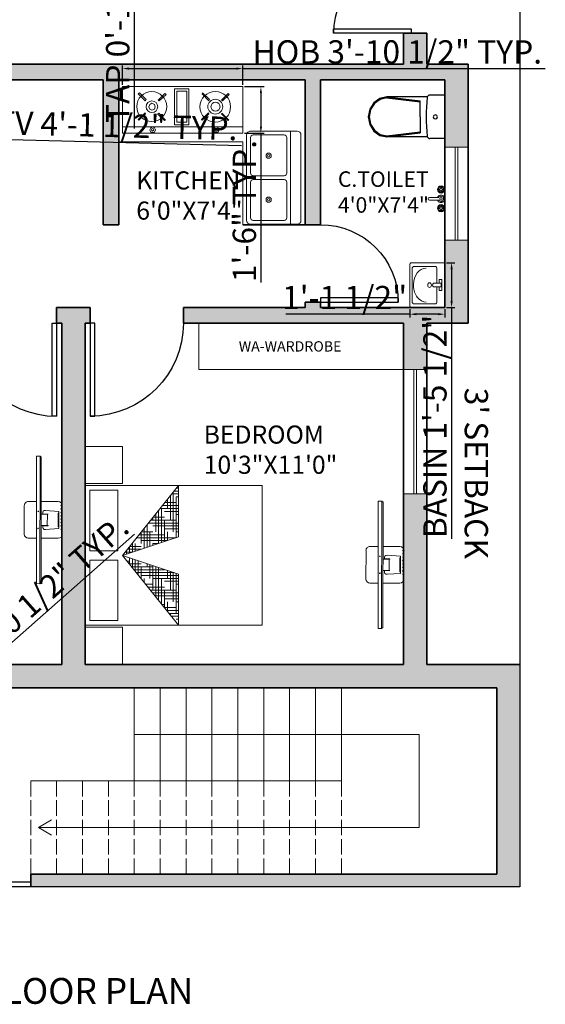
# Model space of a CAD drawing. Units: inches. Extents: x 2831 to 4250, y 1103 to 1797.
# Tile 2 of 15: x 3610 to 3813, y 1197 to 1578. Entities that reach past the tile are written whole.
import ezdxf

# ---------------------------------------------------------------- set-up
doc = ezdxf.new("R2010")
doc.units = ezdxf.units.IN
doc.linetypes.add('ACAD_ISO02W100', pattern=[15, 12, -3])
for name, color, linetype, lineweight in [('A-ANNO-DIMS', 2, 'Continuous', 18), ('A-ANNO-TEXT', 7, 'Continuous', 18), ('A-ANNO-TITL', 7, 'Continuous', 25), ('A-AREA-IDEN', 7, 'Continuous', 18), ('A-DOOR', 4, 'Continuous', 25), ('A-EQPM', 8, 'Continuous', 18), ('A-FLOR-CASE', 9, 'Continuous', 18), ('A-FLOR-STRS', 7, 'Continuous', 18), ('A-FLOR-STRS-HIDN', 8, 'ACAD_ISO02W100', 18), ('A-FLOR-STRS-IDEN', 1, 'Continuous', 18), ('A-WALL', 7, 'Continuous', 35), ('A-WALL-PATT', 252, 'Continuous', 13), ('C-PROP', 7, 'Continuous', 25), ('furn', 8, 'Continuous', 18), ('window', 130, 'Continuous', 18), ('Сантехника', 9, 'Continuous', 18)]:
    doc.layers.add(name, color=color, linetype=linetype, lineweight=lineweight)
doc.layers.add('SANTEH', color=7, linetype='Continuous')
doc.styles.get("Standard").update_dxf_attribs({"font": 'arial.ttf'})
doc.dimstyles.new('ISO-25', dxfattribs={"dimtxt": 9, "dimasz": 2.5, "dimexe": 1.25, "dimexo": 0.625, "dimtad": 1, "dimdec": 1, "dimlunit": 3, "dimtxsty": 'Standard', "dimcen": 2.5, "dimadec": 0, "dimazin": 0, "dimtfac": 1, "dimtdec": 1, "dimtmove": 0, "dimatfit": 3, "dimfxl": 1, "dimarcsym": 0})

# ---------------------------------------------------------------- blocks, each defined once
blk = doc.blocks.new('*U3')
for p, q in [((0, 0), (0, -6)), ((36, 0), (36, -6))]:
    blk.add_line(p, q)
blk.add_lwpolyline([(0, 0), (0, 36), (1.75, 36), (1.75, 0)], close=True)
blk.add_arc((0, 0), 36, 0, 90)
blk = doc.blocks.new('*U4')
for p, q in [((0, 0), (0, -6)), ((30, 0), (30, -6))]:
    blk.add_line(p, q)
blk.add_lwpolyline([(0, 0), (0, 30), (1.75, 30), (1.75, 0)], close=True)
blk.add_arc((0, 0), 30, 0, 90)
blk = doc.blocks.new('gas 1')
for points in [[(35.93, -1.87), (35.93, 0), (0, 0), (0, -1.87)], [(8.12, -0.94), (8.44, -1.56), (8.91, -1.87), (9.53, -1.56), (9.84, -0.94), (9.53, -0.31), (8.91, -0.16), (8.44, -0.31)], [(8.59, -0.94), (8.75, -1.25), (8.91, -1.41), (9.22, -1.25), (9.37, -0.94), (9.22, -0.78), (8.91, -0.62), (8.75, -0.78)], [(19.84, -13.28), (15.47, -13.28), (15.47, -2.5), (19.84, -2.5)], [(27.03, -0.94), (27.34, -1.56), (27.97, -1.87), (28.59, -1.56), (28.75, -0.94), (28.59, -0.31), (27.97, -0.16), (27.34, -0.31)], [(27.5, -0.94), (27.65, -1.25), (27.97, -1.41), (28.28, -1.25), (28.28, -0.94), (28.28, -0.62), (27.97, -0.62), (27.65, -0.62)], [(4.84, -3.91), (4.69, -4.06), (6.72, -6.09), (6.87, -5.78)], [(12.81, -3.91), (12.5, -3.75), (10.47, -5.78), (10.78, -5.94)], [(19.22, -12.5), (16.25, -12.5), (16.25, -3.28), (19.22, -3.28)], [(23.75, -3.91), (23.59, -4.06), (25.62, -6.09), (25.78, -5.78)], [(31.71, -3.91), (31.56, -3.75), (29.53, -5.78), (29.68, -5.94)], [(7.81, -7.81), (8.12, -8.59), (8.75, -8.91), (9.53, -8.59), (9.69, -7.81), (9.53, -7.19), (8.75, -6.87), (8.12, -7.19)], [(7.03, -10), (6.72, -9.69), (4.69, -11.72), (5, -12.03)], [(12.97, -11.56), (10.94, -9.69), (10.62, -9.84), (12.65, -11.87)], [(23.75, -11.72), (23.9, -12.03), (25.93, -10), (25.78, -9.69)], [(31.87, -11.56), (29.84, -9.69), (29.53, -9.84), (31.56, -11.87)]]:
    blk.add_lwpolyline(points, close=True)
blk.add_lwpolyline([(35.93, -1.87), (35.93, -13.9), (0, -13.9), (0, -1.87)])
for centre, radius in [((8.7, -7.92), 4.48), ((27.7, -7.86), 4.58), ((27.69, -7.89), 2.22), ((8.77, -7.89), 1.74), ((27.76, -7.89), 1.35)]:
    blk.add_circle(centre, radius)
blk = doc.blocks.new('Sink-double - 36 in top')
for p, q in [((-18, -4), (18, -4)), ((-0.75, -18.5), (-0.75, -6.5)), ((0.75, -6.5), (0.75, -18.5))]:
    blk.add_line(p, q)
for points in [[(-16.5, 0), (16.5, 0)], [(-18, -19.5), (-18, -1.5)], [(18, -1.5), (18, -19.5)], [(-16.5, -18.5), (-16.5, -6.5)], [(-15.5, -5.5), (-1.75, -5.5)], [(1.75, -5.5), (15.5, -5.5)], [(16.5, -6.5), (16.5, -18.5)], [(16.5, -21), (-16.5, -21)], [(-1.75, -19.5), (-15.5, -19.5)], [(15.5, -19.5), (1.75, -19.5)]]:
    blk.add_lwpolyline(points)
for centre, radius in [((-8.5, -12.5), 1), ((-8.5, -12.5), 0.5), ((8.5, -12.5), 1), ((8.5, -12.5), 0.5)]:
    blk.add_circle(centre, radius)
for centre, radius, start, end in [((-16.5, -1.5), 1.5, 90, 180), ((16.5, -1.5), 1.5, 0, 90), ((-15.5, -6.5), 1, 90, 180), ((-1.75, -6.5), 1, 0, 90), ((1.75, -6.5), 1, 90, 180), ((15.5, -6.5), 1, 0, 90), ((-15.5, -18.5), 1, 180, 270), ((-1.75, -18.5), 1, 270, 0), ((1.75, -18.5), 1, 180, 270), ((15.5, -18.5), 1, 270, 0), ((-16.5, -19.5), 1.5, 180, 270), ((16.5, -19.5), 1.5, 270, 0)]:
    blk.add_arc(centre, radius, start, end)
blk = doc.blocks.new('WC 2 Symb_109')
at = {"layer": 'SANTEH'}
for p, q in [((0, 0), (0, 380)), ((0, 380), (132.4, 380)), ((153.6, 364.9), (506.8, 364.9)), ((506.3, 364.9), (215.7, 330.9)), ((506.3, 356), (215.7, 322)), ((215.7, 190), (215.7, 330.9)), ((215.7, 190), (215.7, 49.1)), ((153.8, 15.1), (506.8, 15.1)), ((506.3, 24), (215.7, 58)), ((506.3, 15.1), (215.7, 49.1)), ((0, 0), (132.4, 0))]:
    blk.add_line(p, q, dxfattribs=at)
for points in [[(154.6, 360.1), (153.9, 364.1), (152.3, 367.9), (150.2, 371.3), (147.4, 374.3), (144.1, 376.7), (140.5, 378.5), (136.5, 379.6), (132.4, 380)], [(154.6, 19.7), (158.6, 62.1), (161.4, 104.7), (163.1, 147.3), (163.7, 189.9), (163.1, 232.5), (161.4, 275.1), (158.6, 317.7), (154.6, 360.1)], [(506.3, 24), (565.5, 36.6), (615.7, 72.6), (649.2, 126.5), (661, 190), (649.2, 253.5), (615.7, 307.4), (565.5, 343.4), (506.3, 356)], [(506.8, 15.1), (569.2, 28.4), (622.2, 66.3), (657.6, 123.1), (670, 190), (657.6, 256.9), (622.2, 313.7), (569.2, 351.6), (506.8, 364.9)], [(132.4, 0), (136.5, 0.4), (140.4, 1.5), (144.1, 3.2), (147.3, 5.6), (150.1, 8.6), (152.3, 12), (153.8, 15.7), (154.6, 19.7)]]:
    blk.add_lwpolyline(points, dxfattribs=at)
blk.add_lwpolyline([(83.6, 208.5), (70.4, 203.1), (64.9, 190), (70.4, 176.9), (83.6, 171.5), (96.8, 176.9), (102.2, 190), (96.8, 203.1)], close=True, dxfattribs=at)
blk = doc.blocks.new('Rac7')
at = {"color": 0}
for p, q in [((-39501, -24232), (-39501, -23830)), ((-39474, -23808), (-38988, -23808)), ((-39032, -23838), (-39430, -23838)), ((-39221, -23855), (-39241, -23855)), ((-38961, -23830), (-38961, -24232)), ((-39457, -23859), (-39457, -24115)), ((-39005, -24115), (-39005, -23859)), ((-39005, -23859), (-39005, -23859)), ((-39253, -24186), (-39253, -24094)), ((-39209, -24186), (-39209, -24094)), ((-39430, -24136), (-39253, -24136)), ((-39297, -24164), (-39253, -24164)), ((-39297, -24194), (-39297, -24164)), ((-39165, -24194), (-39297, -24194)), ((-39253, -24186), (-39209, -24186)), ((-39209, -24136), (-39032, -24136)), ((-39209, -24164), (-39165, -24164)), ((-39165, -24164), (-39165, -24194)), ((-38961, -24232), (-39501, -24232))]:
    blk.add_line(p, q, dxfattribs=at)
at = {"color": 0, "extrusion": (0, 0, -1)}
for centre, major_axis, start_param, end_param in [((-39474, -23830), (-27, 0), 0, 1.570796), ((-39430, -23859), (-27, 0), 0, 1.570796), ((-39241, -24007), (-194, 0), 0, 1.570796), ((-39221, -24007), (-194, 0), 1.570796, 3.141593), ((-39032, -23859), (-27, 0), 1.570796, 3.141593), ((-38988, -23830), (-27, 0), 1.570796, 3.141593), ((-39231, -24104), (-25.3, 0), 0.552816, 2.588777), ((-39430, -24115), (-27, 0), -1.570796, 0), ((-39032, -24115), (-27, 0), -3.141593, -1.570796)]:
    blk.add_ellipse(centre, major_axis=major_axis, ratio=0.785714, start_param=start_param, end_param=end_param, dxfattribs=at)
blk.add_ellipse((-39231, -24048), major_axis=(-27.9, 0), ratio=0.785714, dxfattribs=at)
blk = doc.blocks.new('Faucet - Bathroom top')
for p, q in [((-4.107, 0.125), (-4.375, 0.125)), ((-3.75, 0.4788), (-3.75, 0.75)), ((-3.5, 0.482), (-3.5, 0.75)), ((-3.1461, 0.125), (-2.875, 0.125)), ((3.143, 0.125), (2.875, 0.125)), ((3.5, 0.4788), (3.5, 0.75)), ((3.75, 0.482), (3.75, 0.75)), ((4.1039, 0.125), (4.375, 0.125)), ((-4.1039, -0.125), (-4.375, -0.125)), ((-3.75, -0.4821), (-3.75, -0.75)), ((-3.5, -0.4789), (-3.5, -0.75)), ((-3.143, -0.125), (-2.875, -0.125)), ((-0.5, -0.8639), (-0.5, -4.5)), ((0.5, -4.5), (0.5, -0.8631)), ((3.1461, -0.125), (2.875, -0.125)), ((3.5, -0.4821), (3.5, -0.75)), ((3.75, -0.4789), (3.75, -0.75)), ((4.107, -0.125), (4.375, -0.125))]:
    blk.add_line(p, q)
for centre, radius in [((-3.625, 0), 1.375), ((-4.625, 0), 0.2795), ((-3.625, 0), 0.5), ((-3.625, 1), 0.2795), ((-2.625, 0), 0.2795), ((0, 0), 0.5), ((3.625, 0), 1.375), ((2.625, 0), 0.2795), ((3.625, 0), 0.5), ((3.625, 1), 0.2795), ((4.625, 0), 0.2795), ((-3.625, -1), 0.2795), ((3.625, -1), 0.2795)]:
    blk.add_circle(centre, radius)
for centre, radius, start, end in [((-3.625, 0), 1, 105.2407, 164.2093), ((-3.625, 0), 1, 16.44125, 74.07887), ((0, 0), 1.5, 289.6514, 250.3603), ((0, 0), 1, 300.3431, 239.7554), ((3.625, 0), 1, 106.12, 164.0884), ((3.625, 0), 1, 16.23422, 73.90469), ((-3.625, 0), 1, 196.2342, 253.9047), ((-3.625, 0), 1, 286.12, 344.0884), ((3.625, 0), 1, 196.4413, 254.0789), ((3.625, 0), 1, 285.2407, 344.2093), ((0, -4.5), 0.5, 180, 0)]:
    blk.add_arc(centre, radius, start, end)
blk = doc.blocks.new('*X18')
at = {"color": 0}
for p, q in [((20.25, 14.812), (20.277, 14.812)), ((20.124, 14.688), (20.25, 14.688)), ((20.125, 14.5), (20.125, 14.689)), ((20.149, 14.719), (20.277, 14.719)), ((20.156, 14.625), (20.156, 14.728)), ((20.174, 14.75), (20.277, 14.75)), ((20.188, 14.75), (20.188, 14.767)), ((20.199, 14.781), (20.277, 14.781)), ((20.25, 14.319), (20.25, 14.75)), ((20.062, 14.257), (20.062, 14.612)), ((20.094, 14.375), (20.094, 14.65)), ((20.098, 14.656), (20.125, 14.656)), ((20.125, 14.594), (20.277, 14.594)), ((20.219, 14.309), (20.219, 14.625)), ((20.25, 14.625), (20.277, 14.625)), ((19.973, 14.5), (20.25, 14.5)), ((19.998, 14.531), (20.277, 14.531)), ((20, 14.237), (20, 14.5)), ((20.023, 14.562), (20.277, 14.562)), ((20.031, 14.247), (20.031, 14.573)), ((20.188, 14.299), (20.188, 14.5)), ((19.875, 14.25), (19.875, 14.379)), ((19.906, 14.375), (19.906, 14.417)), ((19.922, 14.438), (20, 14.438)), ((19.948, 14.469), (20.125, 14.469)), ((19.969, 14.226), (19.969, 14.375)), ((20, 14.375), (20.277, 14.375)), ((20.125, 14.406), (20.277, 14.406)), ((20.156, 14.288), (20.156, 14.375)), ((20.25, 14.438), (20.277, 14.438)), ((19.781, 14.164), (19.781, 14.262)), ((19.797, 14.281), (20.125, 14.281)), ((19.812, 14.174), (19.812, 14.301)), ((19.822, 14.312), (20.229, 14.312)), ((19.844, 14.185), (19.844, 14.34)), ((19.875, 14.344), (20.277, 14.344)), ((19.721, 14.188), (19.75, 14.188)), ((19.746, 14.219), (19.875, 14.219)), ((19.75, 14.154), (19.75, 14.223)), ((19.772, 14.25), (20, 14.25)), ((19.938, 14.216), (19.938, 14.25)), ((19.702, 14.094), (19.779, 14.094)), ((19.719, 14.073), (19.719, 14.114)), ((19.727, 14.062), (19.873, 14.062)), ((19.75, 14.034), (19.75, 14.103)), ((19.781, 13.995), (19.781, 14.093)), ((19.812, 14), (19.812, 14.082)), ((19.906, 13.84), (19.906, 14.051)), ((19.752, 14.031), (19.875, 14.031)), ((19.875, 13.878), (19.875, 14)), ((19.875, 13.969), (20.156, 13.969)), ((19.938, 13.801), (19.938, 14.041)), ((19.969, 13.875), (19.969, 14.031)), ((20, 14), (20, 14.02)), ((20, 14), (20.061, 14)), ((20.062, 13.645), (20.062, 14)), ((20.094, 13.625), (20.094, 13.989)), ((20.125, 13.75), (20.125, 13.979)), ((20.156, 13.875), (20.156, 13.969)), ((19.827, 13.938), (20.25, 13.938)), ((19.853, 13.906), (20.125, 13.906)), ((19.878, 13.875), (20, 13.875)), ((20.031, 13.684), (20.031, 13.875)), ((20.125, 13.844), (20.277, 13.844)), ((20.219, 13.451), (20.219, 13.875)), ((20.25, 13.5), (20.25, 13.937)), ((20.25, 13.875), (20.277, 13.875)), ((19.953, 13.781), (20.277, 13.781)), ((19.978, 13.75), (20.25, 13.75)), ((20, 13.812), (20.277, 13.812)), ((20, 13.723), (20, 13.75)), ((20.188, 13.49), (20.188, 13.75)), ((20.003, 13.719), (20.125, 13.719)), ((20.079, 13.625), (20.277, 13.625)), ((20.125, 13.656), (20.277, 13.656)), ((20.156, 13.529), (20.156, 13.625)), ((20.25, 13.688), (20.277, 13.688)), ((20.104, 13.594), (20.277, 13.594)), ((20.129, 13.562), (20.25, 13.562)), ((20.205, 13.469), (20.277, 13.469)), ((20.23, 13.438), (20.277, 13.438)), ((20.25, 13.5), (20.277, 13.5)), ((20.255, 13.406), (20.277, 13.406))]:
    blk.add_line(p, q, dxfattribs=at)
blk = doc.blocks.new('MAT-P02')
for p, q in [((-1.17, 0), (-1.17, -0.4)), ((-1.17, 0), (-0.77, 0)), ((-0.77, 0), (-0.77, -0.4)), ((-0.75, 0), (0.75, 0)), ((-0.75, 0), (-0.75, -1.9)), ((0.75, 0), (0.75, -1.9)), ((0.77, 0), (1.17, 0)), ((0.77, 0), (0.77, -0.4)), ((1.17, 0), (1.17, -0.4)), ((-0.7, -0.05), (-0.7, -0.35)), ((-0.7, -0.05), (-0.05, -0.05)), ((-0.05, -0.35), (-0.05, -0.05)), ((0.05, -0.05), (0.7, -0.05)), ((0.05, -0.35), (0.05, -0.05)), ((0.7, -0.05), (0.7, -0.35)), ((-1.17, -0.4), (-0.77, -0.4)), ((-0.75, -1.003), (0, -0.4)), ((0, -0.4), (-0.75, -1.003)), ((-0.7, -0.35), (-0.05, -0.35)), ((0, -0.4), (-0.2, -1.003)), ((0, -0.4), (0.2, -1.003)), ((0, -0.4), (0.75, -1.003)), ((0.05, -0.35), (0.7, -0.35)), ((0.77, -0.4), (1.17, -0.4)), ((-0.75, -1.003), (-0.2, -1.003)), ((0.2, -1.003), (0.75, -1.003)), ((0.75, -1.9), (-0.75, -1.9))]:
    blk.add_line(p, q)
at = {"xscale": -1, "rotation": 90}
blk.add_blockref('*X18', (14.128, 19.274), dxfattribs=at)
blk = doc.blocks.new('TV')
at = {"color": 0}
for p, q in [((3967.27, 1784.85), (3967.05, 1784.65)), ((3967.76, 1763.68), (3967.54, 1763.86))]:
    blk.add_line(p, q, dxfattribs=at)
at = {"layer": 'window'}
for p, q in [((3967.54, 1763.86), (3967.05, 1784.65)), ((3964.41, 1777.23), (3967.22, 1777.3)), ((3968.01, 1777.32), (3969.36, 1777.35)), ((3966.53, 1775.82), (3964.33, 1775.61)), ((3964.34, 1775.34), (3964.45, 1775.34)), ((3964.34, 1775.31), (3964.43, 1775.32)), ((3966.14, 1775.2), (3967.01, 1775.22)), ((3966.14, 1775.18), (3967.27, 1775.2)), ((3966.14, 1775.18), (3966.14, 1775.2)), ((3966.3, 1773.29), (3966.26, 1775.18)), ((3964.39, 1773.06), (3964.48, 1773.06)), ((3964.39, 1773.04), (3964.5, 1773.04)), ((3966.61, 1772.66), (3964.4, 1772.77)), ((3966.19, 1773.28), (3967.31, 1773.31)), ((3966.19, 1773.26), (3967.05, 1773.28)), ((3966.19, 1773.26), (3966.19, 1773.28)), ((3964.55, 1771.15), (3967.36, 1771.22)), ((3968.15, 1771.24), (3969.5, 1771.27))]:
    blk.add_line(p, q, dxfattribs=at)
for points in [[(3968.33, 1763.69), (3967.83, 1784.86), (3967.27, 1784.85), (3967.76, 1763.68), (3968.33, 1763.69)], [(3963.86, 1771.81), (3963.75, 1776.54)], [(3970.16, 1771.96), (3970.05, 1776.69)], [(3964.4, 1772.77), (3964.33, 1775.61)], [(3964.48, 1773.06), (3964.43, 1775.32)], [(3964.5, 1773.04), (3964.45, 1775.34)]]:
    blk.add_lwpolyline(points, dxfattribs=at)
for points in [[(3966.53, 1775.82, -0.263666), (3966.93, 1775.69), (3967, 1775.57), (3967.01, 1775.22)], [(3966.61, 1772.66, 0.263666), (3967, 1772.81), (3967.06, 1772.93), (3967.05, 1773.28)]]:
    blk.add_lwpolyline(points, format="xyb", dxfattribs=at)
for centre, radius in [((3963.91, 1775.73), 0.0679), ((3963.93, 1775.17), 0.0679), ((3963.94, 1774.6), 0.0679), ((3967.77, 1775.68), 0.0451), ((3963.95, 1774.04), 0.0679), ((3963.97, 1773.48), 0.0679), ((3963.98, 1772.92), 0.0679), ((3967.83, 1772.86), 0.0451), ((3963.99, 1772.35), 0.0679), ((3964.01, 1771.79), 0.0679)]:
    blk.add_circle(centre, radius, dxfattribs=at)
for centre, start, end in [((3964.42, 1776.56), 91.3414, 181.3414), ((3969.38, 1776.67), 1.3414, 91.3414), ((3964.53, 1771.83), 181.3414, 271.3414), ((3969.49, 1771.94), 271.3414, 1.3414)]:
    blk.add_arc(centre, 0.676, start, end, dxfattribs=at)
blk = doc.blocks.new('WIN-36IN')
for p, q in [((0, 36), (9, 36)), ((4, 0), (4, 36)), ((5, 0), (5, 36)), ((0, 0), (9, 0))]:
    blk.add_line(p, q)
blk = doc.blocks.new('WIN-48IN')
for p, q in [((9, 48), (0, 48)), ((4, 0), (4, 48)), ((5, 0), (5, 48)), ((9, 0), (0, 0))]:
    blk.add_line(p, q)
blk = doc.blocks.new('STAIR-TRAVEL-ARROW')
for points in [[(37, 39), (147, 39), (147, 3), (0, 3)], [(5, 0), (0, 3), (5, 6)]]:
    blk.add_lwpolyline(points)
blk = doc.blocks.new('*D81')
at = {"layer": 'A-ANNO-DIMS', "color": 0, "lineweight": -2, "transparency": 16777216}
for p, q in [((3547.26, 1539.7), (3547.06, 1531.68)), ((3596.55, 1538.45), (3596.35, 1530.43)), ((3549.59, 1532.87), (3593.88, 1531.74)), ((3596.38, 1531.68), (3695.71, 1529.15))]:
    blk.add_line(p, q, dxfattribs=at)
at = {"layer": 'A-ANNO-DIMS', "color": 0, "transparency": 16777216}
for points in [[(3549.6, 1533.28), (3549.58, 1532.45), (3547.09, 1532.93)], [(3593.89, 1532.16), (3593.87, 1531.32), (3596.38, 1531.68)]]:
    blk.add_solid(points, dxfattribs=at)
at = {"layer": 'Defpoints', "color": 0, "transparency": 16777216}
for p in [(3547.28, 1540.32), (3596.57, 1539.07), (3596.38, 1531.68)]:
    blk.add_point(p, dxfattribs=at)
at = {"layer": 'A-ANNO-DIMS', "color": 0, "transparency": 16777216, "insert": (3647.43, 1535.66), "char_height": 9, "attachment_point": 5, "rotation": 358.5431}
blk.add_mtext('TV 4\'-1 1/2" TYP.', dxfattribs=at)
blk = doc.blocks.new('*D87')
at = {"layer": 'A-ANNO-DIMS', "color": 0, "lineweight": -2, "transparency": 16777216}
for p, q in [((3649.73, 1552.52), (3649.73, 1560.11)), ((3652.23, 1558.86), (3693.68, 1558.86)), ((3696.18, 1552.52), (3696.18, 1560.11)), ((3696.18, 1558.86), (3813.01, 1558.86))]:
    blk.add_line(p, q, dxfattribs=at)
at = {"layer": 'A-ANNO-DIMS', "color": 0, "transparency": 16777216}
for points in [[(3652.23, 1559.28), (3652.23, 1558.44), (3649.73, 1558.86)], [(3693.68, 1559.28), (3693.68, 1558.44), (3696.18, 1558.86)]]:
    blk.add_solid(points, dxfattribs=at)
at = {"layer": 'Defpoints', "color": 0, "transparency": 16777216}
for p in [(3696.18, 1558.86), (3649.73, 1551.89), (3696.18, 1551.89)]:
    blk.add_point(p, dxfattribs=at)
at = {"layer": 'A-ANNO-DIMS', "color": 0, "transparency": 16777216, "insert": (3755.85, 1564.14), "char_height": 9, "attachment_point": 5}
blk.add_mtext('HOB 3\'-10 1/2" TYP.', dxfattribs=at)
blk = doc.blocks.new('*D88')
at = {"layer": 'A-ANNO-DIMS', "color": 0, "lineweight": -2, "transparency": 16777216}
for p, q in [((3696.81, 1551.89), (3704.4, 1551.89)), ((3703.15, 1549.39), (3703.15, 1536.42)), ((3696.81, 1533.92), (3704.4, 1533.92)), ((3703.15, 1533.92), (3703.15, 1476.16))]:
    blk.add_line(p, q, dxfattribs=at)
at = {"layer": 'A-ANNO-DIMS', "color": 0, "transparency": 16777216}
for points in [[(3702.73, 1549.39), (3703.57, 1549.39), (3703.15, 1551.89)], [(3702.73, 1536.42), (3703.57, 1536.42), (3703.15, 1533.92)]]:
    blk.add_solid(points, dxfattribs=at)
at = {"layer": 'Defpoints', "color": 0, "transparency": 16777216}
for p in [(3696.18, 1551.89), (3696.18, 1533.92), (3703.15, 1533.92)]:
    blk.add_point(p, dxfattribs=at)
at = {"layer": 'A-ANNO-DIMS', "color": 0, "transparency": 16777216, "insert": (3697.93, 1503.79), "char_height": 9, "attachment_point": 5, "rotation": 90}
blk.add_mtext('1\'-6" TYP.', dxfattribs=at)
blk = doc.blocks.new('*D91')
at = {"layer": 'A-ANNO-DIMS', "color": 0, "lineweight": -2, "transparency": 16777216}
for p, q in [((3655.1, 1639.51), (3652.98, 1639.51)), ((3654.23, 1637.01), (3654.23, 1632.01)), ((3655.1, 1629.51), (3652.98, 1629.51)), ((3654.23, 1629.51), (3654.23, 1535.73))]:
    blk.add_line(p, q, dxfattribs=at)
at = {"layer": 'A-ANNO-DIMS', "color": 0, "transparency": 16777216}
for points in [[(3653.81, 1637.01), (3654.64, 1637.01), (3654.23, 1639.51)], [(3653.81, 1632.01), (3654.64, 1632.01), (3654.23, 1629.51)]]:
    blk.add_solid(points, dxfattribs=at)
at = {"layer": 'Defpoints', "color": 0, "transparency": 16777216}
for p in [(3655.73, 1639.51), (3654.23, 1629.51), (3655.73, 1629.51)]:
    blk.add_point(p, dxfattribs=at)
at = {"layer": 'A-ANNO-DIMS', "color": 0, "transparency": 16777216, "insert": (3649.01, 1581.37), "char_height": 9, "attachment_point": 5, "rotation": 90}
blk.add_mtext('TAP 0\'-10" TYP.', dxfattribs=at)
blk = doc.blocks.new('*D94')
at = {"layer": 'A-ANNO-DIMS', "color": 0, "lineweight": -2, "transparency": 16777216}
for p, q in [((3590.07, 1322.17), (3654.36, 1378.87)), ((3591.91, 1320.08), (3589.24, 1323.11)), ((3575.11, 1308.98), (3588.2, 1320.52)), ((3575.08, 1305.23), (3572.41, 1308.26))]:
    blk.add_line(p, q, dxfattribs=at)
at = {"layer": 'A-ANNO-DIMS', "color": 0, "transparency": 16777216}
for points in [[(3587.92, 1320.83), (3588.47, 1320.2), (3590.07, 1322.17)], [(3574.84, 1309.29), (3575.39, 1308.66), (3573.24, 1307.32)]]:
    blk.add_solid(points, dxfattribs=at)
at = {"layer": 'Defpoints', "color": 0, "transparency": 16777216}
for p in [(3590.07, 1322.17), (3592.33, 1319.61), (3575.5, 1304.76)]:
    blk.add_point(p, dxfattribs=at)
at = {"layer": 'A-ANNO-DIMS', "color": 0, "transparency": 16777216, "insert": (3619.66, 1355.31), "char_height": 9, "attachment_point": 5, "rotation": 41.4119}
blk.add_mtext('1\'-10 1/2" TYP.', dxfattribs=at)
blk = doc.blocks.new('*D97')
at = {"layer": 'A-ANNO-DIMS', "color": 0, "lineweight": -2, "transparency": 16777216}
for p, q in [((3774.85, 1483.81), (3778.07, 1483.81)), ((3776.82, 1481.31), (3776.82, 1469.01)), ((3774.85, 1466.51), (3778.07, 1466.51)), ((3776.82, 1466.51), (3776.82, 1377.04))]:
    blk.add_line(p, q, dxfattribs=at)
at = {"layer": 'A-ANNO-DIMS', "color": 0, "transparency": 16777216}
for points in [[(3776.4, 1481.31), (3777.24, 1481.31), (3776.82, 1483.81)], [(3776.4, 1469.01), (3777.24, 1469.01), (3776.82, 1466.51)]]:
    blk.add_solid(points, dxfattribs=at)
at = {"layer": 'Defpoints', "color": 0, "transparency": 16777216}
for p in [(3774.23, 1483.81), (3774.23, 1466.51), (3776.82, 1466.51)]:
    blk.add_point(p, dxfattribs=at)
at = {"layer": 'A-ANNO-DIMS', "color": 0, "transparency": 16777216, "insert": (3771.54, 1420.53), "char_height": 9, "attachment_point": 5, "rotation": 90}
blk.add_mtext('BASIN 1\'-5 1/2"', dxfattribs=at)
blk = doc.blocks.new('*D98')
at = {"layer": 'A-ANNO-DIMS', "color": 0, "lineweight": -2, "transparency": 16777216}
for p, q in [((3760.64, 1465.89), (3760.64, 1462.67)), ((3774.23, 1465.89), (3774.23, 1462.67)), ((3760.64, 1463.92), (3712.84, 1463.92)), ((3771.73, 1463.92), (3763.14, 1463.92))]:
    blk.add_line(p, q, dxfattribs=at)
at = {"layer": 'A-ANNO-DIMS', "color": 0, "transparency": 16777216}
for points in [[(3763.14, 1464.34), (3763.14, 1463.5), (3760.64, 1463.92)], [(3771.73, 1464.34), (3771.73, 1463.5), (3774.23, 1463.92)]]:
    blk.add_solid(points, dxfattribs=at)
at = {"layer": 'Defpoints', "color": 0, "transparency": 16777216}
for p in [(3760.64, 1466.51), (3774.23, 1466.51), (3760.64, 1463.92)]:
    blk.add_point(p, dxfattribs=at)
at = {"layer": 'A-ANNO-DIMS', "color": 0, "transparency": 16777216, "insert": (3735.49, 1469.2), "char_height": 9, "attachment_point": 5}
blk.add_mtext('1\'-1 1/2"', dxfattribs=at)

msp = doc.modelspace()

# ---------------------------------------------------------------- hatches: boundary and pattern name
at = {"layer": 'A-WALL-PATT'}
h = msp.add_hatch(color=256, dxfattribs=at)
h.dxf.hatch_style = 1
h.paths.add_polyline_path([(3479.23, 1418.51), (3488.23, 1418.51), (3488.23, 1426.81), (3488.23, 1460.51), (3588.23, 1460.51), (3588.23, 1466.51), (3488.23, 1466.51), (3488.23, 1470.51), (3479.23, 1470.51)])
h.paths.add_polyline_path([(3488.23, 1506.51), (3488.23, 1512.51), (3479.23, 1512.51), (3479.23, 1506.51)])
h.paths.add_polyline_path([(3488.23, 1370.51), (3479.23, 1370.51), (3479.23, 1319.51), (3521.23, 1319.51), (3521.23, 1328.51), (3488.23, 1328.51)])
h.paths.add_polyline_path([(3794.23, 1319.51), (3794.23, 1247.51), (3614.23, 1247.51), (3614.23, 1242.51), (3803.23, 1242.51), (3803.23, 1328.51), (3767.23, 1328.51), (3767.23, 1394.51), (3758.23, 1394.51), (3758.23, 1328.51), (3635.23, 1328.51), (3635.23, 1460.51), (3637.23, 1460.51), (3637.23, 1466.51), (3624.23, 1466.51), (3624.23, 1460.51), (3626.23, 1460.51), (3626.23, 1328.51), (3593.23, 1328.51), (3593.23, 1319.51)])
h.paths.add_polyline_path([(3758.23, 1460.51), (3758.23, 1442.51), (3767.23, 1442.51), (3767.23, 1460.51), (3783.23, 1460.51), (3783.23, 1492.51), (3774.23, 1492.51), (3774.23, 1466.51), (3761.32, 1466.51), (3726.23, 1466.51), (3726.23, 1468.51), (3720.23, 1468.51), (3720.23, 1466.51), (3673.23, 1466.51), (3673.23, 1460.51)])
h.paths.add_polyline_path([(3597.63, 1698.24), (3687.22, 1698.24), (3687.22, 1717.46), (3597.63, 1717.46)], flags=9)
h.paths.add_polyline_path([(3776.75, 1438.29), (3776.75, 1360.77), (3795.97, 1360.77), (3795.97, 1438.29)], flags=25)
h.paths.add_polyline_path([(3453.37, 1482.95), (3453.37, 1401.85), (3472.59, 1401.85), (3472.59, 1482.95)], flags=9)
h.paths.add_polyline_path([(3506.21, 1267.1), (3560.71, 1267.1), (3560.71, 1293.71), (3506.21, 1293.71)], flags=9)
h.paths.add_polyline_path([(3760.5, 1579.7), (3798.74, 1579.7), (3798.74, 1602.51), (3760.5, 1602.51)], flags=9)
h.paths.add_polyline_path([(3617, 1637.95), (3659.12, 1637.95), (3659.12, 1660.76), (3617, 1660.76)], flags=9)
h.paths.add_polyline_path([(3679.39, 1612.63), (3728.46, 1612.63), (3728.46, 1639.25), (3679.39, 1639.25)], flags=9)
h.paths.add_polyline_path([(3731.07, 1499.72), (3773.19, 1499.72), (3773.19, 1522.53), (3731.07, 1522.53)], flags=9)
h.paths.add_polyline_path([(3652.82, 1496.49), (3701.95, 1496.49), (3701.95, 1523.1), (3652.82, 1523.1)], flags=9)
h.paths.add_polyline_path([(3550.37, 1510.97), (3604.5, 1510.97), (3604.5, 1537.58), (3550.37, 1537.58)], flags=9)
h.paths.add_polyline_path([(3514.45, 1612.63), (3570.67, 1612.63), (3570.67, 1639.25), (3514.45, 1639.25)], flags=9)
h = msp.add_hatch(color=256, dxfattribs=at)
h.dxf.hatch_style = 1
h.paths.add_polyline_path([(3783.23, 1560.51), (3767.23, 1560.51), (3767.23, 1572.51), (3761.23, 1572.51), (3758.23, 1572.51), (3758.23, 1560.51), (3488.23, 1560.51), (3488.23, 1562.51), (3485.23, 1562.51), (3479.23, 1562.51), (3479.23, 1552.51), (3485.23, 1552.51), (3488.23, 1552.51), (3488.23, 1554.51), (3642.23, 1554.51), (3642.23, 1498.51), (3648.23, 1498.51), (3648.23, 1554.51), (3720.23, 1554.51), (3720.23, 1498.51), (3726.23, 1498.51), (3726.23, 1554.51), (3774.23, 1554.51), (3774.23, 1528.51), (3783.23, 1528.51)])
h.paths.add_polyline_path([(3767.23, 1689.51), (3728.23, 1689.51), (3728.23, 1680.51), (3758.23, 1680.51), (3758.23, 1602.51), (3767.23, 1602.51)])
h.paths.add_polyline_path([(3680.23, 1689.51), (3656.23, 1689.51), (3656.23, 1680.51), (3662.23, 1680.51), (3662.23, 1608.51), (3644.23, 1608.51), (3644.23, 1602.51), (3668.23, 1602.51), (3668.23, 1680.51), (3680.23, 1680.51)])
h.paths.add_polyline_path([(3620.23, 1689.51), (3584.23, 1689.51), (3584.23, 1680.51), (3608.23, 1680.51), (3608.23, 1602.51), (3614.23, 1602.51), (3614.23, 1608.51), (3614.23, 1638.51), (3614.23, 1680.51), (3620.23, 1680.51)])
h.paths.add_polyline_path([(3512.23, 1689.51), (3479.23, 1689.51), (3479.23, 1665.51), (3488.23, 1665.51), (3488.23, 1680.51), (3512.23, 1680.51)])
h.paths.add_polyline_path([(3488.23, 1617.51), (3479.23, 1617.51), (3479.23, 1602.51), (3485.23, 1602.51), (3488.23, 1602.51)])

# ---------------------------------------------------------------- linework, layer by layer
at = {"layer": 'A-FLOR-CASE'}
for p, q in [((3648.23, 1530.51), (3696.23, 1530.51)), ((3696.23, 1498.51), (3696.23, 1530.51)), ((3679.23, 1442.51), (3679.23, 1460.51)), ((3679.23, 1442.51), (3758.23, 1442.51))]:
    msp.add_line(p, q, dxfattribs=at)
at = {"layer": 'A-FLOR-STRS'}
for p, q in [((3654.23, 1319.51), (3654.23, 1283.51)), ((3664.23, 1319.51), (3664.23, 1283.51)), ((3674.23, 1319.51), (3674.23, 1283.51)), ((3684.23, 1319.51), (3684.23, 1283.51)), ((3694.23, 1319.51), (3694.23, 1283.51)), ((3704.23, 1319.51), (3704.23, 1283.51)), ((3714.23, 1319.51), (3714.23, 1283.51)), ((3724.23, 1319.51), (3724.23, 1283.51)), ((3734.23, 1319.51), (3734.23, 1283.51)), ((3734.23, 1283.51), (3614.23, 1283.51))]:
    msp.add_line(p, q, dxfattribs=at)
at = {"layer": 'A-FLOR-STRS-HIDN', "ltscale": 0.5}
for p, q in [((3614.23, 1283.51), (3614.23, 1247.51)), ((3624.23, 1283.51), (3624.23, 1247.51)), ((3634.23, 1283.51), (3634.23, 1247.51)), ((3644.23, 1283.51), (3644.23, 1247.51)), ((3654.23, 1283.51), (3654.23, 1247.51)), ((3664.23, 1283.51), (3664.23, 1247.51)), ((3674.23, 1283.51), (3674.23, 1247.51)), ((3684.23, 1283.51), (3684.23, 1247.51)), ((3694.23, 1283.51), (3694.23, 1247.51)), ((3704.23, 1283.51), (3704.23, 1247.51)), ((3714.23, 1283.51), (3714.23, 1247.51)), ((3724.23, 1283.51), (3724.23, 1247.51)), ((3734.23, 1283.51), (3734.23, 1247.51))]:
    msp.add_line(p, q, dxfattribs=at)
at = {"layer": 'A-WALL'}
for p, q in [((3758.23, 1572.51), (3767.23, 1572.51)), ((3758.23, 1572.51), (3758.23, 1560.51)), ((3767.23, 1572.51), (3767.23, 1560.51)), ((3488.23, 1560.51), (3758.23, 1560.51)), ((3767.23, 1560.51), (3783.23, 1560.51)), ((3783.23, 1460.51), (3783.23, 1560.51)), ((3488.23, 1554.51), (3642.23, 1554.51)), ((3642.23, 1498.51), (3642.23, 1554.51)), ((3648.23, 1554.51), (3720.23, 1554.51)), ((3648.23, 1498.51), (3648.23, 1554.51)), ((3720.23, 1498.51), (3720.23, 1554.51)), ((3726.23, 1554.51), (3774.23, 1554.51)), ((3726.23, 1498.51), (3726.23, 1554.51)), ((3774.23, 1466.51), (3774.23, 1554.51)), ((3642.23, 1498.51), (3648.23, 1498.51)), ((3696.23, 1498.51), (3726.23, 1498.51)), ((3624.23, 1460.51), (3624.23, 1466.51)), ((3624.23, 1466.51), (3637.23, 1466.51)), ((3637.23, 1460.51), (3637.23, 1466.51)), ((3673.23, 1460.51), (3673.23, 1466.51)), ((3673.23, 1466.51), (3720.23, 1466.51)), ((3720.23, 1466.51), (3720.23, 1468.51)), ((3720.23, 1468.51), (3726.23, 1468.51)), ((3726.23, 1466.51), (3726.23, 1468.51)), ((3726.23, 1466.51), (3774.23, 1466.51)), ((3624.23, 1460.51), (3626.23, 1460.51)), ((3626.23, 1328.51), (3626.23, 1460.51)), ((3635.23, 1328.51), (3635.23, 1460.51)), ((3635.23, 1460.51), (3637.23, 1460.51)), ((3673.23, 1460.51), (3758.23, 1460.51)), ((3758.23, 1460.51), (3758.23, 1328.51)), ((3767.23, 1460.51), (3767.23, 1328.51)), ((3767.23, 1460.51), (3783.23, 1460.51)), ((3488.23, 1328.51), (3626.23, 1328.51)), ((3635.23, 1328.51), (3758.23, 1328.51)), ((3767.23, 1328.51), (3803.23, 1328.51)), ((3479.23, 1319.51), (3794.23, 1319.51)), ((3794.23, 1319.51), (3794.23, 1247.51)), ((3614.23, 1247.51), (3794.23, 1247.51)), ((3614.23, 1247.51), (3614.23, 1242.51))]:
    msp.add_line(p, q, dxfattribs=at)
at = {"layer": 'C-PROP'}
msp.add_line((3445.23, 1244.51), (3614.23, 1244.51), dxfattribs=at)
msp.add_lwpolyline([(3443.23, 1722.51), (3803.23, 1722.51), (3803.23, 1242.51), (3443.23, 1242.51)], close=True, dxfattribs=at)

# ---------------------------------------------------------------- block references
at = {"layer": 'A-DOOR'}
for name, p, rotation in [('*U4', (3761.23, 1572.51), 90), ('*U3', (3624.23, 1460.51), 180)]:
    msp.add_blockref(name, p, dxfattribs=dict(at, rotation=rotation))
at = {"layer": 'A-DOOR', "xscale": -1}
for name, p, rotation in [('*U4', (3726.23, 1468.51), 270), ('*U3', (3637.23, 1460.51), 180)]:
    msp.add_blockref(name, p, dxfattribs=dict(at, rotation=rotation))
at = {"layer": 'A-EQPM'}
for name, p, xscale, yscale, zscale, rotation in [('gas 1', (3649.73, 1533.92), -1.292580420916565, 1.292580420916565, 1.292580420916565, 180), ('TV', (12953.45, 5277.57), 2.327319231123021, 2.327319231123021, 2.327319231123021, 178.5430845181612), ('TV', (13085.45, 5260.23), 2.327319231123021, 2.327319231123021, 2.327319231123021, 178.5430845181612)]:
    msp.add_blockref(name, p, dxfattribs=dict(at, xscale=xscale, yscale=yscale, zscale=zscale, rotation=rotation))
at = {"layer": 'A-FLOR-STRS-IDEN'}
msp.add_blockref('STAIR-TRAVEL-ARROW', (3617.23, 1262.51), dxfattribs=at)
at = {"layer": 'furn', "xscale": 36.03633950593442, "yscale": 36.03633950593442, "zscale": 36.03633950593442, "rotation": 90}
msp.add_blockref('MAT-P02', (3635.23, 1370.68), dxfattribs=at)
at = {"layer": 'window'}
for name, p in [('WIN-36IN', (3774.23, 1492.51)), ('WIN-48IN', (3758.23, 1394.51))]:
    msp.add_blockref(name, p, dxfattribs=at)
at = {"layer": 'Сантехника'}
for name, p, xscale, yscale, zscale, rotation in [('WC 2 Symb_109', (3774.23, 1548.59), 0.0441898926459964, 0.0441898926459964, 0.0441898926459964, 180), ('Rac7', (2997.17, 217.14), -0.0320670790485951, 0.0320670790485951, 0.0320670790485951, 90)]:
    msp.add_blockref(name, p, dxfattribs=dict(at, xscale=xscale, yscale=yscale, zscale=zscale, rotation=rotation))
at = {"layer": 'Сантехника', "xscale": -1, "rotation": 270}
msp.add_blockref('Sink-double - 36 in top', (3718.64, 1516.69), dxfattribs=at)
at = {"layer": 'Сантехника', "rotation": 270}
msp.add_blockref('Faucet - Bathroom top', (3772.73, 1508.51), dxfattribs=at)

# ---------------------------------------------------------------- texts
at = {"layer": 'A-ANNO-TEXT', "insert": (3694.6, 1453.48), "char_height": 4, "attachment_point": 1}
msp.add_mtext_dynamic_manual_height_columns('WA-WARDROBE', width=29.5334, gutter_width=12.5, heights=[0], dxfattribs=at)
at = {"layer": 'A-ANNO-TEXT', "insert": (3790.87, 1435.5), "char_height": 9, "attachment_point": 1, "rotation": 270}
msp.add_mtext_dynamic_manual_height_columns("{\\fTimes New Roman|b0|i0|c0|p18;3' SETBACK}", width=81.5075, gutter_width=12.5, heights=[0], dxfattribs=at)
at = {"layer": 'A-ANNO-TITL', "insert": (3556.39, 1207.34), "char_height": 10, "attachment_point": 1}
msp.add_mtext_dynamic_manual_height_columns('{\\fTimes New Roman|b0|i0|c0|p18;FIRST FLOOR PLAN}', width=196.2607, gutter_width=12.5, heights=[0], dxfattribs=at)
at = {"layer": 'A-AREA-IDEN', "attachment_point": 1}
for s, insert, char_height in [('{\\fTimes New Roman|b0|i0|c0|p18;KITCHEN\\P6\'0"X7\'4"}', (3655.01, 1519.14), 7), ('{\\fTimes New Roman|b0|i0|c0|p18;C.TOILET\\P4\'0"X7\'4"}', (3732.89, 1519.14), 6), ('{\\fTimes New Roman|b0|i0|c0|p18;BEDROOM\\P10\'3"X11\'0"}', (3681.05, 1420.89), 7)]:
    msp.add_mtext_dynamic_manual_height_columns(s, width=81.5075, gutter_width=12.5, heights=[0], dxfattribs=dict(at, insert=insert, char_height=char_height))

# ---------------------------------------------------------------- dimensions: what is measured, and where the dimension line sits
at = {"layer": 'A-ANNO-DIMS'}
for base, p1, p2, angle, text, picture, middle in [((3654.23, 1629.51), (3655.73, 1639.51), (3655.73, 1629.51), 270, 'TAP <> TYP.', '*D91', (3649.01, 1581.37)), ((3596.38, 1531.68), (3547.28, 1540.32), (3596.57, 1539.07), 358.5431, 'TV <> TYP.', '*D81', (3647.43, 1535.66)), ((3703.15, 1533.92), (3696.18, 1551.89), (3696.18, 1533.92), 270, '<> TYP.', '*D88', (3697.93, 1503.79)), ((3776.82, 1466.51), (3774.23, 1483.81), (3774.23, 1466.51), 270, 'BASIN <>', '*D97', (3771.54, 1420.53)), ((3590.07, 1322.17), (3575.5, 1304.76), (3592.33, 1319.61), 41.4119, '<> TYP.', '*D94', (3619.66, 1355.31))]:
    dim = msp.add_linear_dim(base=base, p1=p1, p2=p2, angle=angle, text=text, dimstyle='ISO-25', override={"dimdec": 1, "dimlfac": 1, "dimrnd": 0, "dimzin": 1, "dimdsep": 46, "dimlunit": 4, "dimfrac": 2}, dxfattribs=at)
    dim.commit()
    dim.dimension.update_dxf_attribs({"geometry": picture, "text_midpoint": middle})
dim = msp.add_linear_dim(base=(3696.1815, 1558.8587), p1=(3649.7349, 1551.8917), p2=(3696.1815, 1551.8917), text='HOB <> TYP.', dimstyle='ISO-25', override={"dimdec": 1, "dimlfac": 1, "dimrnd": 0, "dimzin": 1, "dimdsep": 46, "dimlunit": 4, "dimfrac": 2}, dxfattribs=at)
dim.commit()
dim.dimension.update_dxf_attribs({"geometry": '*D87', "text_midpoint": (3755.845, 1564.1433)})
dim = msp.add_linear_dim(base=(3760.64, 1463.92), p1=(3774.23, 1466.51), p2=(3760.64, 1466.51), angle=180, dimstyle='ISO-25', override={"dimdec": 1, "dimlfac": 1, "dimrnd": 0, "dimzin": 1, "dimdsep": 46, "dimlunit": 4, "dimfrac": 2}, dxfattribs=at)
dim.commit()
dim.dimension.update_dxf_attribs({"geometry": '*D98', "text_midpoint": (3735.49, 1469.2)})

doc.saveas('drawing.dxf')
